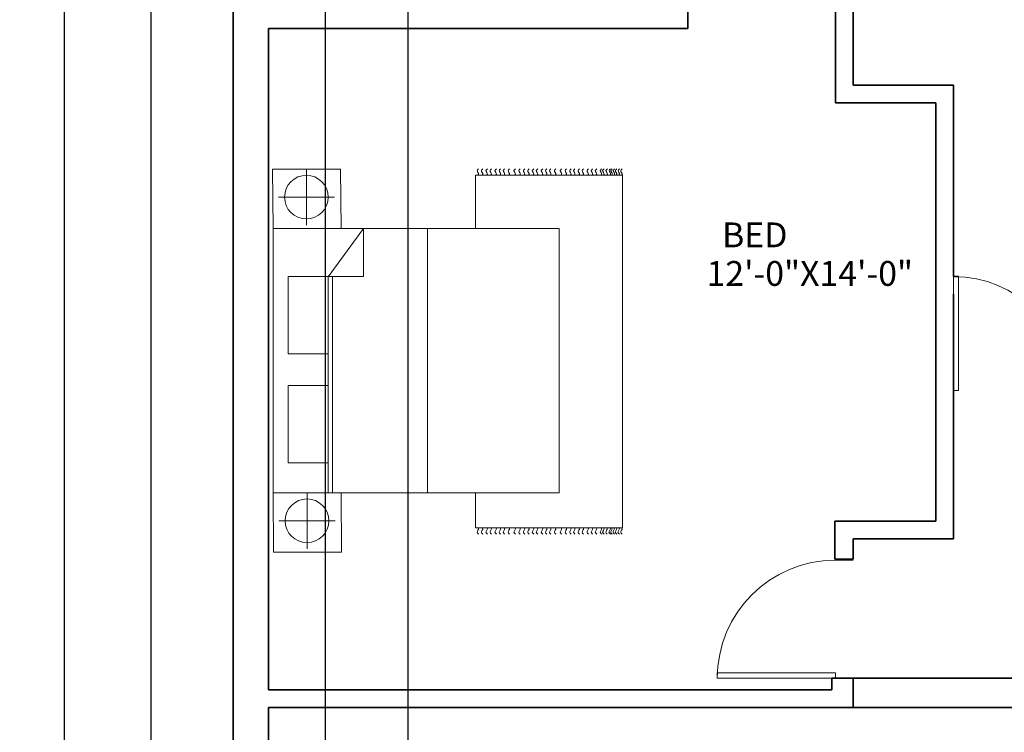
# Model space of a CAD drawing. Units: inches. Extents: x 79 to 8696167, y -3690578 to 147.
# Tile 4 of 10: x 79 to 329, y -223 to -42. Entities that reach past the tile are written whole.
import ezdxf

# ---------------------------------------------------------------- set-up
doc = ezdxf.new("R2010")
doc.units = ezdxf.units.IN
doc.header["$MEASUREMENT"] = 0
doc.layers.get('0').update_dxf_attribs({"color": 253})
for name, color, linetype, lineweight in [('A-ANNO-DIMS', 2, 'Continuous', 18), ('A-AREA-IDEN', 7, 'Continuous', 18), ('A-DOOR', 4, 'Continuous', 18), ('C-PROP', 7, 'Continuous', 35), ('furniture', 30, 'Continuous', 18), ('walls', 8, 'Continuous', 35)]:
    doc.layers.add(name, color=color, linetype=linetype, lineweight=lineweight)
doc.styles.get("Standard").update_dxf_attribs({"font": 'arial.ttf'})
doc.dimstyles.get("Standard").update_dxf_attribs({"dimtxt": 6, "dimasz": 0.18, "dimexe": 0.18, "dimexo": 0.0625, "dimgap": 0.09, "dimtad": 0, "dimtih": 1, "dimtoh": 1, "dimzin": 0, "dimdsep": 46, "dimlunit": 3, "dimtxsty": 'Standard', "dimcen": 0.09, "dimadec": 0, "dimazin": 0, "dimtfac": 1, "dimtofl": 0, "dimtmove": 0, "dimatfit": 3, "dimfxl": 1, "dimtolj": 1, "dimtzin": 0, "dimarcsym": 0})

# ---------------------------------------------------------------- blocks, each defined once
blk = doc.blocks.new('CARPET')
at = {"layer": 'furniture'}
for p, q in [((-51.53, -98.11), (-51.53, -55.12)), ((-51.53, -55.12), (-41.27, -55.12)), ((36, -55.12), (51.55, -55.12)), ((51.55, -55.12), (51.55, -98.11)), ((51.55, -98.11), (-51.53, -98.11))]:
    blk.add_line(p, q, dxfattribs=at)
for points, knots in [([(-53.37, -55.99), (-53.22, -55.8), (-52.9, -55.41), (-52.34, -55.8), (-51.89, -56.08), (-51.65, -55.91), (-51.53, -55.83)], [0, 0, 0, 0, 0.653278, 1.290138, 1.740457, 2.114451, 2.114451, 2.114451, 2.114451]), ([(-53.37, -57.26), (-53.22, -57.07), (-52.9, -56.67), (-52.34, -57.07), (-51.89, -57.35), (-51.65, -57.17), (-51.53, -57.1)], [0, 0, 0, 0, 0.653278, 1.290138, 1.740457, 2.114451, 2.114451, 2.114451, 2.114451]), ([(53.37, -55.99), (53.22, -55.8), (52.9, -55.41), (52.34, -55.8), (51.89, -56.08), (51.65, -55.91), (51.53, -55.83)], [0, 0, 0, 0, 0.653278, 1.290138, 1.740457, 2.114451, 2.114451, 2.114451, 2.114451]), ([(53.37, -57.26), (53.22, -57.07), (52.9, -56.67), (52.34, -57.07), (51.89, -57.35), (51.65, -57.17), (51.53, -57.1)], [0, 0, 0, 0, 0.653278, 1.290138, 1.740457, 2.114451, 2.114451, 2.114451, 2.114451]), ([(-53.37, -58.59), (-53.22, -58.4), (-52.9, -58.01), (-52.34, -58.4), (-51.89, -58.68), (-51.65, -58.5), (-51.53, -58.43)], [0, 0, 0, 0, 0.653278, 1.290138, 1.740457, 2.114451, 2.114451, 2.114451, 2.114451]), ([(-53.37, -59.78), (-53.22, -59.58), (-52.9, -59.19), (-52.34, -59.58), (-51.89, -59.86), (-51.65, -59.69), (-51.53, -59.61)], [0, 0, 0, 0, 0.653278, 1.290138, 1.740457, 2.114451, 2.114451, 2.114451, 2.114451]), ([(53.37, -58.59), (53.22, -58.4), (52.9, -58.01), (52.34, -58.4), (51.89, -58.68), (51.65, -58.5), (51.53, -58.43)], [0, 0, 0, 0, 0.653278, 1.290138, 1.740457, 2.114451, 2.114451, 2.114451, 2.114451]), ([(53.37, -59.78), (53.22, -59.58), (52.9, -59.19), (52.34, -59.58), (51.89, -59.86), (51.65, -59.69), (51.53, -59.61)], [0, 0, 0, 0, 0.653278, 1.290138, 1.740457, 2.114451, 2.114451, 2.114451, 2.114451]), ([(-53.37, -61.22), (-53.22, -61.02), (-52.9, -60.63), (-52.34, -61.02), (-51.89, -61.3), (-51.65, -61.13), (-51.53, -61.05)], [0, 0, 0, 0, 0.653278, 1.290138, 1.740457, 2.114451, 2.114451, 2.114451, 2.114451]), ([(-53.37, -62.44), (-53.22, -62.25), (-52.9, -61.86), (-52.34, -62.25), (-51.89, -62.53), (-51.65, -62.36), (-51.53, -62.28)], [0, 0, 0, 0, 0.653278, 1.290138, 1.740457, 2.114451, 2.114451, 2.114451, 2.114451]), ([(-53.37, -63.63), (-53.22, -63.43), (-52.9, -63.04), (-52.34, -63.43), (-51.89, -63.72), (-51.65, -63.54), (-51.53, -63.46)], [0, 0, 0, 0, 0.653278, 1.290138, 1.740457, 2.114451, 2.114451, 2.114451, 2.114451]), ([(53.37, -61.22), (53.22, -61.02), (52.9, -60.63), (52.34, -61.02), (51.89, -61.3), (51.65, -61.13), (51.53, -61.05)], [0, 0, 0, 0, 0.653278, 1.290138, 1.740457, 2.114451, 2.114451, 2.114451, 2.114451]), ([(53.37, -62.44), (53.22, -62.25), (52.9, -61.86), (52.34, -62.25), (51.89, -62.53), (51.65, -62.36), (51.53, -62.28)], [0, 0, 0, 0, 0.653278, 1.290138, 1.740457, 2.114451, 2.114451, 2.114451, 2.114451]), ([(53.37, -63.63), (53.22, -63.43), (52.9, -63.04), (52.34, -63.43), (51.89, -63.72), (51.65, -63.54), (51.53, -63.46)], [0, 0, 0, 0, 0.653278, 1.290138, 1.740457, 2.114451, 2.114451, 2.114451, 2.114451]), ([(-53.37, -65.07), (-53.22, -64.87), (-52.9, -64.48), (-52.34, -64.87), (-51.89, -65.15), (-51.65, -64.98), (-51.53, -64.9)], [0, 0, 0, 0, 0.653278, 1.290138, 1.740457, 2.114451, 2.114451, 2.114451, 2.114451]), ([(53.37, -65.07), (53.22, -64.87), (52.9, -64.48), (52.34, -64.87), (51.89, -65.15), (51.65, -64.98), (51.53, -64.9)], [0, 0, 0, 0, 0.653278, 1.290138, 1.740457, 2.114451, 2.114451, 2.114451, 2.114451]), ([(-53.37, -66.76), (-53.22, -66.56), (-52.9, -66.17), (-52.34, -66.56), (-51.89, -66.84), (-51.65, -66.67), (-51.53, -66.59)], [0, 0, 0, 0, 0.653278, 1.290138, 1.740457, 2.114451, 2.114451, 2.114451, 2.114451]), ([(-53.37, -68.2), (-53.22, -68), (-52.9, -67.61), (-52.34, -68), (-51.89, -68.28), (-51.65, -68.11), (-51.53, -68.03)], [0, 0, 0, 0, 0.653278, 1.290138, 1.740457, 2.114451, 2.114451, 2.114451, 2.114451]), ([(53.37, -66.76), (53.22, -66.56), (52.9, -66.17), (52.34, -66.56), (51.89, -66.84), (51.65, -66.67), (51.53, -66.59)], [0, 0, 0, 0, 0.653278, 1.290138, 1.740457, 2.114451, 2.114451, 2.114451, 2.114451]), ([(53.37, -68.2), (53.22, -68), (52.9, -67.61), (52.34, -68), (51.89, -68.28), (51.65, -68.11), (51.53, -68.03)], [0, 0, 0, 0, 0.653278, 1.290138, 1.740457, 2.114451, 2.114451, 2.114451, 2.114451]), ([(-53.37, -69.53), (-53.22, -69.33), (-52.9, -68.94), (-52.34, -69.33), (-51.89, -69.61), (-51.65, -69.44), (-51.53, -69.36)], [0, 0, 0, 0, 0.653278, 1.290138, 1.740457, 2.114451, 2.114451, 2.114451, 2.114451]), ([(-53.37, -70.79), (-53.22, -70.6), (-52.9, -70.21), (-52.34, -70.6), (-51.89, -70.88), (-51.65, -70.7), (-51.53, -70.63)], [0, 0, 0, 0, 0.653278, 1.290138, 1.740457, 2.114451, 2.114451, 2.114451, 2.114451]), ([(-53.37, -72.12), (-53.22, -71.93), (-52.9, -71.54), (-52.34, -71.93), (-51.89, -72.21), (-51.65, -72.04), (-51.53, -71.96)], [0, 0, 0, 0, 0.653278, 1.290138, 1.740457, 2.114451, 2.114451, 2.114451, 2.114451]), ([(53.37, -69.53), (53.22, -69.33), (52.9, -68.94), (52.34, -69.33), (51.89, -69.61), (51.65, -69.44), (51.53, -69.36)], [0, 0, 0, 0, 0.653278, 1.290138, 1.740457, 2.114451, 2.114451, 2.114451, 2.114451]), ([(53.37, -70.79), (53.22, -70.6), (52.9, -70.21), (52.34, -70.6), (51.89, -70.88), (51.65, -70.7), (51.53, -70.63)], [0, 0, 0, 0, 0.653278, 1.290138, 1.740457, 2.114451, 2.114451, 2.114451, 2.114451]), ([(53.37, -72.12), (53.22, -71.93), (52.9, -71.54), (52.34, -71.93), (51.89, -72.21), (51.65, -72.04), (51.53, -71.96)], [0, 0, 0, 0, 0.653278, 1.290138, 1.740457, 2.114451, 2.114451, 2.114451, 2.114451]), ([(-53.37, -73.31), (-53.22, -73.11), (-52.9, -72.72), (-52.34, -73.11), (-51.89, -73.4), (-51.65, -73.22), (-51.53, -73.14)], [0, 0, 0, 0, 0.653278, 1.290138, 1.740457, 2.114451, 2.114451, 2.114451, 2.114451]), ([(-53.37, -74.75), (-53.22, -74.55), (-52.9, -74.16), (-52.34, -74.55), (-51.89, -74.83), (-51.65, -74.66), (-51.53, -74.58)], [0, 0, 0, 0, 0.653278, 1.290138, 1.740457, 2.114451, 2.114451, 2.114451, 2.114451]), ([(53.37, -73.31), (53.22, -73.11), (52.9, -72.72), (52.34, -73.11), (51.89, -73.4), (51.65, -73.22), (51.53, -73.14)], [0, 0, 0, 0, 0.653278, 1.290138, 1.740457, 2.114451, 2.114451, 2.114451, 2.114451]), ([(53.37, -74.75), (53.22, -74.55), (52.9, -74.16), (52.34, -74.55), (51.89, -74.83), (51.65, -74.66), (51.53, -74.58)], [0, 0, 0, 0, 0.653278, 1.290138, 1.740457, 2.114451, 2.114451, 2.114451, 2.114451]), ([(-53.37, -75.98), (-53.22, -75.78), (-52.9, -75.39), (-52.34, -75.78), (-51.89, -76.06), (-51.65, -75.89), (-51.53, -75.81)], [0, 0, 0, 0, 0.653278, 1.290138, 1.740457, 2.114451, 2.114451, 2.114451, 2.114451]), ([(-53.37, -77.16), (-53.22, -76.96), (-52.9, -76.57), (-52.34, -76.96), (-51.89, -77.25), (-51.65, -77.07), (-51.53, -76.99)], [0, 0, 0, 0, 0.653278, 1.290138, 1.740457, 2.114451, 2.114451, 2.114451, 2.114451]), ([(53.37, -75.98), (53.22, -75.78), (52.9, -75.39), (52.34, -75.78), (51.89, -76.06), (51.65, -75.89), (51.53, -75.81)], [0, 0, 0, 0, 0.653278, 1.290138, 1.740457, 2.114451, 2.114451, 2.114451, 2.114451]), ([(53.37, -77.16), (53.22, -76.96), (52.9, -76.57), (52.34, -76.96), (51.89, -77.25), (51.65, -77.07), (51.53, -76.99)], [0, 0, 0, 0, 0.653278, 1.290138, 1.740457, 2.114451, 2.114451, 2.114451, 2.114451]), ([(-53.37, -78.6), (-53.22, -78.4), (-52.9, -78.01), (-52.34, -78.4), (-51.89, -78.68), (-51.65, -78.51), (-51.53, -78.43)], [0, 0, 0, 0, 0.653278, 1.290138, 1.740457, 2.114451, 2.114451, 2.114451, 2.114451]), ([(-53.37, -80.29), (-53.22, -80.09), (-52.9, -79.7), (-52.34, -80.09), (-51.89, -80.37), (-51.65, -80.2), (-51.53, -80.12)], [0, 0, 0, 0, 0.653278, 1.290138, 1.740457, 2.114451, 2.114451, 2.114451, 2.114451]), ([(53.37, -78.6), (53.22, -78.4), (52.9, -78.01), (52.34, -78.4), (51.89, -78.68), (51.65, -78.51), (51.53, -78.43)], [0, 0, 0, 0, 0.653278, 1.290138, 1.740457, 2.114451, 2.114451, 2.114451, 2.114451]), ([(53.37, -80.29), (53.22, -80.09), (52.9, -79.7), (52.34, -80.09), (51.89, -80.37), (51.65, -80.2), (51.53, -80.12)], [0, 0, 0, 0, 0.653278, 1.290138, 1.740457, 2.114451, 2.114451, 2.114451, 2.114451]), ([(-53.37, -81.73), (-53.22, -81.53), (-52.9, -81.14), (-52.34, -81.53), (-51.89, -81.81), (-51.65, -81.64), (-51.53, -81.56)], [0, 0, 0, 0, 0.653278, 1.290138, 1.740457, 2.114451, 2.114451, 2.114451, 2.114451]), ([(-53.37, -83.06), (-53.22, -82.86), (-52.9, -82.47), (-52.34, -82.86), (-51.89, -83.14), (-51.65, -82.97), (-51.53, -82.89)], [0, 0, 0, 0, 0.653278, 1.290138, 1.740457, 2.114451, 2.114451, 2.114451, 2.114451]), ([(53.37, -81.73), (53.22, -81.53), (52.9, -81.14), (52.34, -81.53), (51.89, -81.81), (51.65, -81.64), (51.53, -81.56)], [0, 0, 0, 0, 0.653278, 1.290138, 1.740457, 2.114451, 2.114451, 2.114451, 2.114451]), ([(53.37, -83.06), (53.22, -82.86), (52.9, -82.47), (52.34, -82.86), (51.89, -83.14), (51.65, -82.97), (51.53, -82.89)], [0, 0, 0, 0, 0.653278, 1.290138, 1.740457, 2.114451, 2.114451, 2.114451, 2.114451]), ([(-53.37, -84.18), (-53.22, -83.99), (-52.9, -83.6), (-52.34, -83.99), (-51.89, -84.27), (-51.65, -84.09), (-51.53, -84.02)], [0, 0, 0, 0, 0.653278, 1.290138, 1.740457, 2.114451, 2.114451, 2.114451, 2.114451]), ([(-53.37, -85.51), (-53.22, -85.32), (-52.9, -84.93), (-52.34, -85.32), (-51.89, -85.6), (-51.65, -85.42), (-51.53, -85.35)], [0, 0, 0, 0, 0.653278, 1.290138, 1.740457, 2.114451, 2.114451, 2.114451, 2.114451]), ([(-53.37, -86.7), (-53.22, -86.5), (-52.9, -86.11), (-52.34, -86.5), (-51.89, -86.78), (-51.65, -86.61), (-51.53, -86.53)], [0, 0, 0, 0, 0.653278, 1.290138, 1.740457, 2.114451, 2.114451, 2.114451, 2.114451]), ([(53.37, -84.18), (53.22, -83.99), (52.9, -83.6), (52.34, -83.99), (51.89, -84.27), (51.65, -84.09), (51.53, -84.02)], [0, 0, 0, 0, 0.653278, 1.290138, 1.740457, 2.114451, 2.114451, 2.114451, 2.114451]), ([(53.37, -85.51), (53.22, -85.32), (52.9, -84.93), (52.34, -85.32), (51.89, -85.6), (51.65, -85.42), (51.53, -85.35)], [0, 0, 0, 0, 0.653278, 1.290138, 1.740457, 2.114451, 2.114451, 2.114451, 2.114451]), ([(53.37, -86.7), (53.22, -86.5), (52.9, -86.11), (52.34, -86.5), (51.89, -86.78), (51.65, -86.61), (51.53, -86.53)], [0, 0, 0, 0, 0.653278, 1.290138, 1.740457, 2.114451, 2.114451, 2.114451, 2.114451]), ([(-53.37, -88.14), (-53.22, -87.94), (-52.9, -87.55), (-52.34, -87.94), (-51.89, -88.22), (-51.65, -88.05), (-51.53, -87.97)], [0, 0, 0, 0, 0.653278, 1.290138, 1.740457, 2.114451, 2.114451, 2.114451, 2.114451]), ([(-53.37, -89.36), (-53.22, -89.17), (-52.9, -88.78), (-52.34, -89.17), (-51.89, -89.45), (-51.65, -89.28), (-51.53, -89.2)], [0, 0, 0, 0, 0.653278, 1.290138, 1.740457, 2.114451, 2.114451, 2.114451, 2.114451]), ([(53.37, -88.14), (53.22, -87.94), (52.9, -87.55), (52.34, -87.94), (51.89, -88.22), (51.65, -88.05), (51.53, -87.97)], [0, 0, 0, 0, 0.653278, 1.290138, 1.740457, 2.114451, 2.114451, 2.114451, 2.114451]), ([(53.37, -89.36), (53.22, -89.17), (52.9, -88.78), (52.34, -89.17), (51.89, -89.45), (51.65, -89.28), (51.53, -89.2)], [0, 0, 0, 0, 0.653278, 1.290138, 1.740457, 2.114451, 2.114451, 2.114451, 2.114451]), ([(-53.37, -90.55), (-53.22, -90.35), (-52.9, -89.96), (-52.34, -90.35), (-51.89, -90.64), (-51.65, -90.46), (-51.53, -90.38)], [0, 0, 0, 0, 0.653278, 1.290138, 1.740457, 2.114451, 2.114451, 2.114451, 2.114451]), ([(-53.37, -91.99), (-53.22, -91.79), (-52.9, -91.4), (-52.34, -91.79), (-51.89, -92.07), (-51.65, -91.9), (-51.53, -91.82)], [0, 0, 0, 0, 0.653278, 1.290138, 1.740457, 2.114451, 2.114451, 2.114451, 2.114451]), ([(53.37, -90.55), (53.22, -90.35), (52.9, -89.96), (52.34, -90.35), (51.9, -90.63), (51.66, -90.47), (51.55, -90.4)], [0, 0, 0, 0, 0.653278, 1.290138, 1.740457, 2.0926, 2.0926, 2.0926, 2.0926]), ([(53.37, -91.99), (53.22, -91.79), (52.9, -91.4), (52.34, -91.79), (51.9, -92.07), (51.66, -91.91), (51.55, -91.83)], [0, 0, 0, 0, 0.653278, 1.290138, 1.740457, 2.0926, 2.0926, 2.0926, 2.0926]), ([(-53.37, -92.69), (-53.22, -92.48), (-52.9, -92.08), (-52.35, -92.49), (-51.89, -92.77), (-51.65, -92.6), (-51.53, -92.52)], [0, 0, 0, 0, 0.663904, 1.307406, 1.757725, 2.131719, 2.131719, 2.131719, 2.131719]), ([(-53.37, -93.61), (-53.22, -93.42), (-52.9, -93.03), (-52.34, -93.42), (-51.89, -93.7), (-51.65, -93.52), (-51.53, -93.45)], [0, 0, 0, 0, 0.653278, 1.290138, 1.740457, 2.114451, 2.114451, 2.114451, 2.114451]), ([(-53.37, -94.55), (-53.22, -94.35), (-52.9, -93.96), (-52.34, -94.35), (-51.89, -94.63), (-51.65, -94.46), (-51.53, -94.38)], [0, 0, 0, 0, 0.653278, 1.290138, 1.740457, 2.114451, 2.114451, 2.114451, 2.114451]), ([(-53.37, -95.05), (-53.22, -94.85), (-52.9, -94.46), (-52.34, -94.85), (-51.89, -95.14), (-51.65, -94.96), (-51.53, -94.88)], [0, 0, 0, 0, 0.653278, 1.290138, 1.740457, 2.114451, 2.114451, 2.114451, 2.114451]), ([(53.37, -92.69), (53.22, -92.49), (52.9, -92.09), (52.34, -92.49), (51.9, -92.77), (51.66, -92.61), (51.55, -92.53)], [0, 0, 0, 0, 0.656792, 1.295826, 1.746145, 2.098292, 2.098292, 2.098292, 2.098292]), ([(53.37, -93.66), (53.22, -93.46), (52.9, -93.07), (52.34, -93.46), (51.9, -93.74), (51.66, -93.58), (51.55, -93.5)], [0, 0, 0, 0, 0.653278, 1.290138, 1.740457, 2.0926, 2.0926, 2.0926, 2.0926]), ([(53.37, -94.59), (53.22, -94.4), (52.9, -94.01), (52.34, -94.4), (51.9, -94.68), (51.66, -94.51), (51.55, -94.44)], [0, 0, 0, 0, 0.653278, 1.290138, 1.740457, 2.0926, 2.0926, 2.0926, 2.0926]), ([(53.37, -95.1), (53.22, -94.9), (52.9, -94.51), (52.34, -94.9), (51.9, -95.18), (51.66, -95.02), (51.55, -94.94)], [0, 0, 0, 0, 0.653278, 1.290138, 1.740457, 2.0926, 2.0926, 2.0926, 2.0926]), ([(-53.37, -95.73), (-53.22, -95.54), (-52.9, -95.15), (-52.34, -95.54), (-51.89, -95.82), (-51.65, -95.65), (-51.53, -95.57)], [0, 0, 0, 0, 0.653278, 1.290138, 1.740457, 2.114451, 2.114451, 2.114451, 2.114451]), ([(-53.37, -96.38), (-53.22, -96.18), (-52.9, -95.79), (-52.34, -96.18), (-51.89, -96.47), (-51.65, -96.29), (-51.53, -96.21)], [0, 0, 0, 0, 0.653278, 1.290138, 1.740457, 2.114451, 2.114451, 2.114451, 2.114451]), ([(-53.37, -97.17), (-53.22, -96.98), (-52.9, -96.59), (-52.34, -96.98), (-51.89, -97.26), (-51.65, -97.08), (-51.53, -97.01)], [0, 0, 0, 0, 0.653278, 1.290138, 1.740457, 2.114451, 2.114451, 2.114451, 2.114451]), ([(-53.37, -97.99), (-53.22, -97.79), (-52.9, -97.4), (-52.34, -97.79), (-51.89, -98.08), (-51.65, -97.9), (-51.53, -97.82)], [0, 0, 0, 0, 0.653278, 1.290138, 1.740457, 2.114451, 2.114451, 2.114451, 2.114451]), ([(53.37, -95.78), (53.22, -95.58), (52.9, -95.19), (52.34, -95.58), (51.89, -95.86), (51.65, -95.69), (51.53, -95.61)], [0, 0, 0, 0, 0.653278, 1.290138, 1.740457, 2.114451, 2.114451, 2.114451, 2.114451]), ([(53.37, -96.43), (53.22, -96.23), (52.9, -95.84), (52.34, -96.23), (51.89, -96.51), (51.65, -96.34), (51.53, -96.26)], [0, 0, 0, 0, 0.653278, 1.290138, 1.740457, 2.114451, 2.114451, 2.114451, 2.114451]), ([(53.37, -97.22), (53.22, -97.02), (52.9, -96.63), (52.34, -97.02), (51.89, -97.3), (51.65, -97.13), (51.53, -97.05)], [0, 0, 0, 0, 0.653278, 1.290138, 1.740457, 2.114451, 2.114451, 2.114451, 2.114451]), ([(53.37, -97.99), (53.22, -97.79), (52.9, -97.4), (52.34, -97.79), (51.89, -98.08), (51.65, -97.9), (51.53, -97.82)], [0, 0, 0, 0, 0.653278, 1.290138, 1.740457, 2.114451, 2.114451, 2.114451, 2.114451])]:
    blk.add_open_spline(points, degree=3, knots=knots, dxfattribs=at)
blk = doc.blocks.new('A$C58D270C6')
at = {"layer": 'furniture'}
for p, q in [((9.09, 124.13), (9.09, 108.87)), ((1.46, 116.5), (16.73, 116.5)), ((14.97, 94.84), (24.62, 107.92)), ((24.62, 94.93), (24.62, 107.92)), ((42.08, 108), (42.08, 36)), ((14.97, 94.93), (24.62, 94.93)), ((14.97, 94.84), (14.97, 36)), ((16.22, 94.93), (16.22, 36)), ((9.25, 36), (9.25, 20.74)), ((1.62, 28.37), (16.88, 28.37))]:
    blk.add_line(p, q, dxfattribs=at)
for points in [[(18.5, 108), (18.34, 124.13), (-0.16, 124.13), (0, 108)], [(0, 108), (77.91, 108), (77.91, 36), (0, 36)], [(4.09, 94.93), (14.97, 94.93), (14.97, 73.83), (4.09, 73.83)], [(4.09, 65.23), (14.97, 65.23), (14.97, 44.13), (4.09, 44.13)], [(18.65, 19.87), (18.5, 36), (0, 36), (0.16, 19.87)]]:
    blk.add_lwpolyline(points, close=True, dxfattribs=at)
for centre in [(9.09, 116.5), (9.25, 28.37)]:
    blk.add_circle(centre, 5.95, dxfattribs=at)
at = {"layer": 'furniture', "xscale": 0.9312884925094044, "yscale": 0.9312884925094044, "zscale": 0.9312884925094044, "rotation": 90}
blk.add_blockref('CARPET', (3.79, 74.47), dxfattribs=at)
blk = doc.blocks.new('*U12')
for p, q in [((0, 0), (0, -6)), ((40, 0), (40, -6))]:
    blk.add_line(p, q)
blk.add_lwpolyline([(0, 0), (0, 40), (1.75, 40), (1.75, 0)], close=True)
blk.add_arc((0, 0), 40, 0, 90)
blk = doc.blocks.new('*D23')
at = {"layer": 'A-ANNO-DIMS', "color": 0, "lineweight": -2, "transparency": 16777216}
for p, q in [((133.38, 99.88), (112.4, 99.88)), ((112.58, 99.7), (112.58, -286.97)), ((112.58, -679.94), (112.58, -293.28)), ((133.38, -680.12), (112.4, -680.12))]:
    blk.add_line(p, q, dxfattribs=at)
at = {"layer": 'A-ANNO-DIMS', "color": 0, "lineweight": 100, "transparency": 16777216}
for points in [[(112.55, 99.7), (112.61, 99.7), (112.58, 99.88)], [(112.55, -679.94), (112.61, -679.94), (112.58, -680.12)]]:
    blk.add_solid(points, dxfattribs=at)
at = {"layer": 'Defpoints', "color": 0, "lineweight": 100, "transparency": 16777216}
for p in [(112.58, 99.88), (133.44, 99.88), (133.44, -680.12)]:
    blk.add_point(p, dxfattribs=at)
at = {"layer": 'A-ANNO-DIMS', "color": 0, "transparency": 16777216, "insert": (112.58, -290.12), "char_height": 6, "attachment_point": 5}
blk.add_mtext("\\A1;65'", dxfattribs=at)
blk = doc.blocks.new('*D56')
at = {"layer": 'A-ANNO-DIMS', "color": 0, "lineweight": -2, "transparency": 16777216}
for p, q in [((133.38, 35.38), (90.36, 35.38)), ((90.54, 35.2), (90.54, -253.97)), ((90.54, -549.44), (90.54, -260.28)), ((133.38, -549.62), (90.36, -549.62))]:
    blk.add_line(p, q, dxfattribs=at)
at = {"layer": 'A-ANNO-DIMS', "color": 0, "lineweight": 100, "transparency": 16777216}
for points in [[(90.51, 35.2), (90.57, 35.2), (90.54, 35.38)], [(90.51, -549.44), (90.57, -549.44), (90.54, -549.62)]]:
    blk.add_solid(points, dxfattribs=at)
at = {"layer": 'Defpoints', "color": 0, "lineweight": 100, "transparency": 16777216}
for p in [(90.54, 35.38), (133.44, 35.38), (133.44, -549.62)]:
    blk.add_point(p, dxfattribs=at)
at = {"layer": 'A-ANNO-DIMS', "color": 0, "transparency": 16777216, "insert": (90.54, -257.12), "char_height": 6, "attachment_point": 5}
blk.add_mtext('\\A1;48\'-9"', dxfattribs=at)
blk = doc.blocks.new('*D59')
at = {"layer": 'A-ANNO-DIMS', "color": 0, "lineweight": -2, "transparency": 16777216}
for p, q in [((156.82, 2.31), (156.82, -723.2)), ((177.82, 2.31), (177.82, -723.2)), ((157, -723.02), (159.53, -723.02)), ((177.64, -723.02), (175.1, -723.02))]:
    blk.add_line(p, q, dxfattribs=at)
at = {"layer": 'A-ANNO-DIMS', "color": 0, "lineweight": 100, "transparency": 16777216}
for points in [[(157, -722.99), (157, -723.05), (156.82, -723.02)], [(177.64, -722.99), (177.64, -723.05), (177.82, -723.02)]]:
    blk.add_solid(points, dxfattribs=at)
at = {"layer": 'Defpoints', "color": 0, "lineweight": 100, "transparency": 16777216}
for p in [(156.82, 2.38), (177.82, 2.38), (177.82, -723.02)]:
    blk.add_point(p, dxfattribs=at)
at = {"layer": 'A-ANNO-DIMS', "color": 0, "transparency": 16777216, "insert": (167.32, -723.02), "char_height": 6, "attachment_point": 5}
blk.add_mtext('\\A1;1\'-9"', dxfattribs=at)

msp = doc.modelspace()

# ---------------------------------------------------------------- linework, layer by layer
at = {"layer": 'C-PROP'}
msp.add_line((133.441, -680.125), (133.441, 99.875), dxfattribs=at)
at = {"layer": 'walls'}
for p, q in [((248.941, -44.125), (248.941, 26.375)), ((286.441, -62.986), (286.441, 26.375)), ((290.941, -58.486), (290.941, 26.375)), ((142.441, -44.125), (248.941, -44.125)), ((142.441, -212.125), (142.441, -44.125)), ((286.441, -58.486), (286.441, -62.986)), ((290.941, -58.486), (316.441, -58.486)), ((316.441, -58.486), (316.441, -107.125)), ((286.441, -62.986), (311.941, -62.986)), ((311.941, -62.986), (311.941, -111.625)), ((316.441, -107.125), (317.709, -107.125)), ((311.941, -111.625), (311.941, -169.266)), ((316.441, -111.625), (316.441, -169.266)), ((311.941, -169.266), (286.309, -169.266)), ((286.309, -169.266), (286.309, -178.922)), ((316.441, -169.266), (316.441, -173.766)), ((316.441, -173.766), (290.941, -173.766)), ((290.941, -178.922), (290.941, -173.766)), ((286.309, -178.922), (290.941, -178.922)), ((285.524, -212.125), (285.524, -209.184)), ((285.524, -209.184), (290.941, -209.184)), ((290.941, -209.184), (290.941, -212.125)), ((290.941, -209.184), (343.419, -209.184)), ((142.441, -212.125), (285.524, -212.125)), ((290.941, -216.625), (290.941, -212.125)), ((142.441, -540.625), (142.441, -216.625)), ((142.441, -216.625), (290.941, -216.625)), ((290.941, -216.625), (343.419, -216.625))]:
    msp.add_line(p, q, dxfattribs=at)

# ---------------------------------------------------------------- block references
at = {"layer": 'A-DOOR', "xscale": 0.7244533731370114, "yscale": 0.7244533731370114, "zscale": 0.7244533731370114}
msp.add_blockref('*U12', (316.441, -136.099), dxfattribs=at)
at = {"layer": 'A-DOOR', "xscale": 0.7498099103642428, "yscale": 0.7498099103642428, "zscale": 0.7498099103642428, "rotation": 90}
msp.add_blockref('*U12', (286.442, -209.184), dxfattribs=at)
at = {"layer": 'furniture', "xscale": 0.9331788672991836, "yscale": 0.9331788672991836, "zscale": 0.9331788672991836}
msp.add_blockref('A$C58D270C6', (143.592, -195.678), dxfattribs=at)

# ---------------------------------------------------------------- texts
at = {"layer": 'A-AREA-IDEN'}
for s, height, p in [('BED', 6.302, (257.661, -99.707)), ('12\'-0"X14\'-0"', 6.30205, (253.718, -109.501))]:
    msp.add_text(s, height=height, dxfattribs=at).set_placement(p)

# ---------------------------------------------------------------- dimensions: what is measured, and where the dimension line sits
at = {"layer": 'A-ANNO-DIMS'}
for base, p1, p2, override, picture, middle in [((112.58, 99.875), (133.441, -680.125), (133.441, 99.875), {"dimclrd": 0, "dimclre": 0, "dimclrt": 0}, '*D23', (112.58, -290.125)), ((90.541, 35.375), (133.441, -549.625), (133.441, 35.375), {"dimdec": 1, "dimlfac": 1, "dimrnd": 0, "dimzin": 1, "dimdsep": 46, "dimlunit": 4, "dimfrac": 2}, '*D56', (90.541, -257.125))]:
    dim = msp.add_linear_dim(base=base, p1=p1, p2=p2, angle=90, dimstyle='Standard', override=override, dxfattribs=at)
    dim.commit()
    dim.dimension.update_dxf_attribs({"geometry": picture, "text_midpoint": middle})
dim = msp.add_linear_dim(base=(177.817, -723.025), p1=(156.817, 2.375), p2=(177.817, 2.375), dimstyle='Standard', override={"dimdec": 1, "dimlfac": 1, "dimrnd": 0, "dimzin": 1, "dimdsep": 46, "dimlunit": 4, "dimfrac": 2}, dxfattribs=at)
dim.commit()
dim.dimension.update_dxf_attribs({"geometry": '*D59', "text_midpoint": (167.317, -723.025)})

doc.saveas('drawing.dxf')
